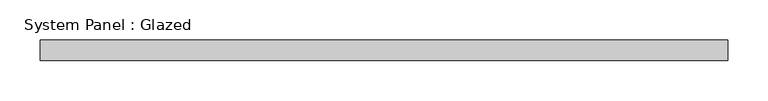
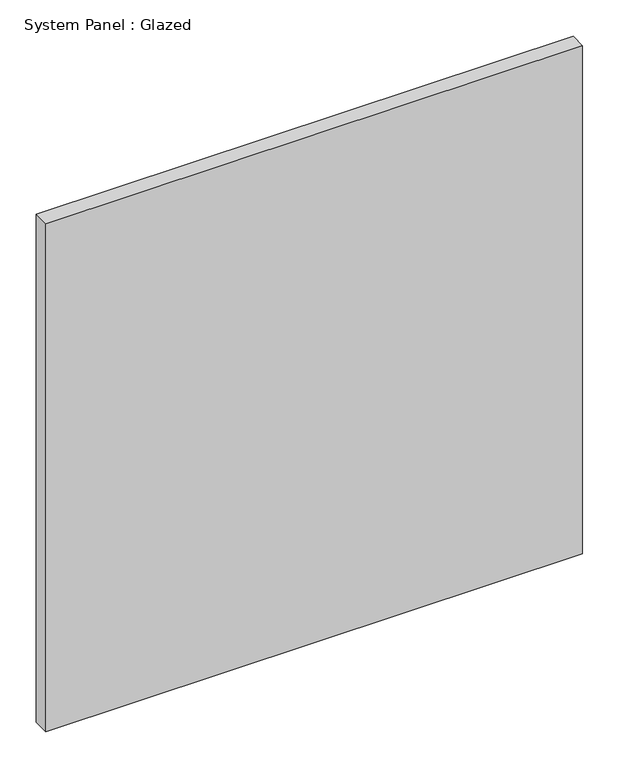
"""IFC4 building model written with IfcOpenShell, lengths in millimetres: plate geometry, System Panel : Glazed."""

from ifc_helpers import new_model, si_unit, origin, origin_with_axes, place, context, project, spatial, polyline, outline, extrude, source, transform, mapped, element, save


def system_panel_glazed_9a5ea490(model_context):
    return source(origin(), model_context, "Body", "SweptSolid", [
        extrude(outline(polyline([(425.45, 19.05), (-425.45, 19.05), (-425.45, 44.45), (425.45, 44.45), (425.45, 19.05)])), origin_with_axes(), (0.0, 0.0, 1.0), 850.9),
    ])


if __name__ == "__main__":
    model = new_model("IFC4")
    model_context = context("Model", 3, world=origin())
    ifc_project = project(units=[si_unit("LENGTHUNIT", "METRE", prefix="MILLI")], contexts=[model_context])
    site = spatial("IfcSite", under=ifc_project)
    building = spatial("IfcBuilding", under=site)
    placement = place(None, origin())
    system_panel_glazed_shape = system_panel_glazed_9a5ea490(model_context)
    element("IfcPlate", 1, ObjectType="System Panel : Glazed", at=placement, inside=building, context=model_context, shape_type="MappedRepresentation", body=[
        mapped(system_panel_glazed_shape, transform((0.0, 0.0, 0.0), x_axis=(1.0, 0.0, 0.0), y_axis=(0.0, 1.0, 0.0), z_axis=(0.0, 0.0, 1.0))),
    ])
    save(model, "model.ifc")

# Revit data of these elements
# Type "System Panel : Glazed"
#   Construction Type Id = "GSP4R"
#   Analytic Construction = "1/8 in Pilkington single glazing"
#   Visual Light Transmittance = 0.9
#   Solar Heat Gain Coefficient = 0.86
#   Heat Transfer Coefficient (U) = 6.7069 W/(m²·K)
# Element 1 (IfcPlate, "System Panel : Glazed")
#   Materials on its faces: "Glass"
# Materials
#   "Glass": class "Glass", colour RGB 0 128 192, transparency 0.75, Description = "Soda Lime Glass", Cost = 0
